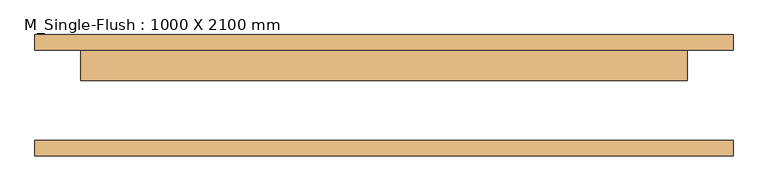
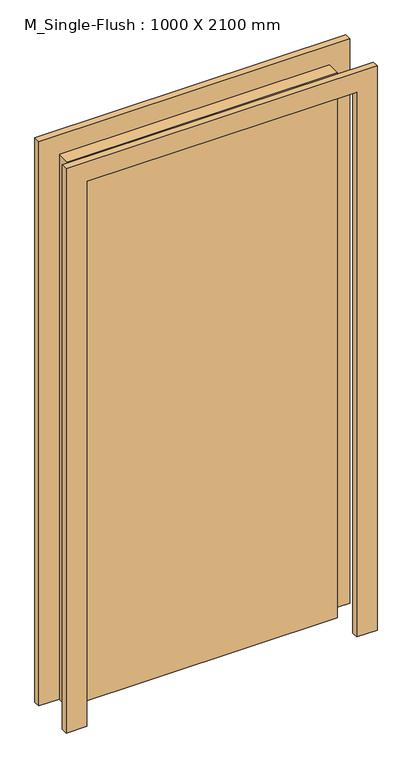
"""IFC4 building model written with IfcOpenShell, lengths in millimetres: door geometry, M_Single-Flush : 1000 X 2100 mm."""

from ifc_helpers import new_model, si_unit, frame, origin, origin_with_axes, place, context, project, spatial, polyline, outline, extrude, source, transform, mapped, element, save


def m_single_flush_1000_x_2100_mm_e4293d47(model_context):
    return source(origin(), model_context, "Body", "SweptSolid", [
        extrude(outline(polyline([(2210.0, -576.0), (0.0, -576.0), (0.0, -500.0), (2134.0, -500.0), (2134.0, 500.0), (0.0, 500.0), (0.0, 576.0), (2210.0, 576.0), (2210.0, -576.0)])), frame((0.0, 75.0, 0.0), z_axis=(0.0, 1.0, 0.0), x_axis=(0.0, 0.0, 1.0)), (0.0, 0.0, 1.0), 25.0),
        extrude(outline(polyline([(2210.0, 576.0), (2210.0, -576.0), (0.0, -576.0), (0.0, -500.0), (2134.0, -500.0), (2134.0, 500.0), (0.0, 500.0), (0.0, 576.0), (2210.0, 576.0)])), frame((0.0, -100.0, 0.0), z_axis=(0.0, 1.0, 0.0), x_axis=(0.0, 0.0, 1.0)), (0.0, 0.0, 1.0), 25.0),
        extrude(outline(polyline([(500.0, 24.0), (-500.0, 24.0), (-500.0, 75.0), (500.0, 75.0), (500.0, 24.0)])), origin_with_axes(), (0.0, 0.0, 1.0), 2134.0),
    ])


if __name__ == "__main__":
    model = new_model("IFC4")
    model_context = context("Model", 3, world=origin())
    ifc_project = project(units=[si_unit("LENGTHUNIT", "METRE", prefix="MILLI")], contexts=[model_context])
    site = spatial("IfcSite", under=ifc_project)
    building = spatial("IfcBuilding", under=site)
    placement = place(None, origin())
    m_single_flush_1000_x_2100_mm_shape = m_single_flush_1000_x_2100_mm_e4293d47(model_context)
    element("IfcDoor", 1, ObjectType="M_Single-Flush : 1000 X 2100 mm", at=placement, inside=building, context=model_context, shape_type="MappedRepresentation", body=[
        mapped(m_single_flush_1000_x_2100_mm_shape, transform((0.0, 0.0, 0.0), x_axis=(1.0, 0.0, 0.0), y_axis=(0.0, 1.0, 0.0), z_axis=(0.0, 0.0, 1.0))),
    ])
    save(model, "model.ifc")

# Revit data of these elements
# Type "M_Single-Flush : 1000 X 2100 mm"
#   Type Mark = "40"
#   Construction Type Id = "MDOOR"
#   Analytic Construction = "Metal"
#   Thickness = 0.051 m
#   Thermal Resistance (R) = 0.270117 (m²·K)/W
#   Heat Transfer Coefficient (U) = 3.7021 W/(m²·K)
#   Height = 2.134 m
#   Trim Projection Ext = 0.025 m
#   Trim Projection Int = 0.025 m
#   Trim Width = 0.076 m
#   Width = 1 m
#   Define Thermal Properties by = 1
#   Door Material = Door - Panel
#   Frame Material = Door - Frame
#   Visual Light Transmittance = 0
#   Solar Heat Gain Coefficient = 0
#   Function = (empty or 0)
#   Wall Closure = (empty or 0)
# Element 1 (IfcDoor, "M_Single-Flush : 1000 X 2100 mm")
#   Materials on its faces: "Door - Frame", "Door - Panel"
# Materials
#   "Door - Panel": class "Wood", colour RGB 210 159 95, transparency 0, Cost = 0
#   "Door - Frame": colour RGB 118 70 51, transparency 0, Cost = 0
